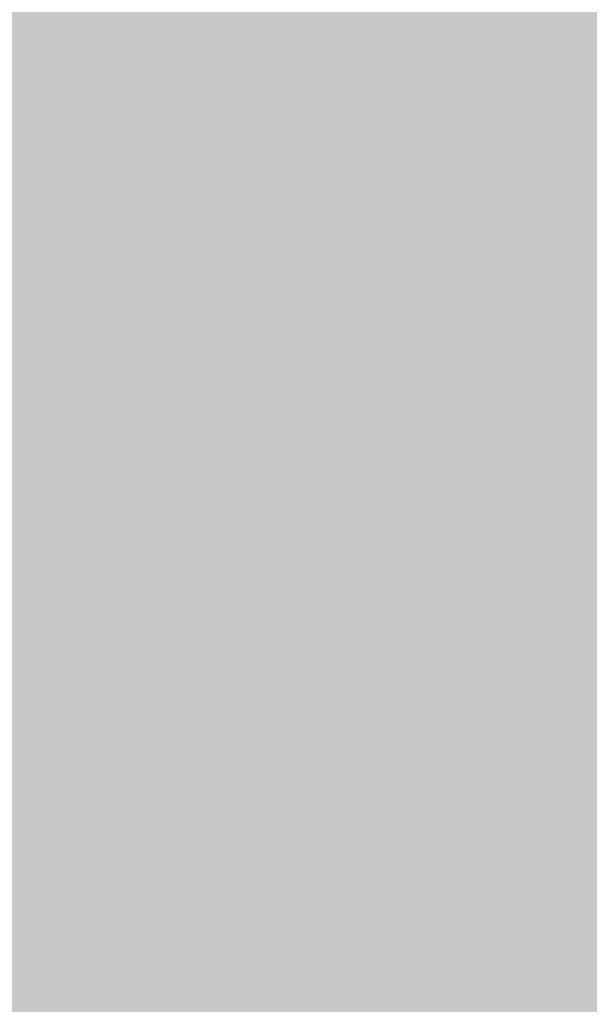
# Model space of a CAD drawing. Units: millimetres. Extents: x -22994 to 29398, y -19990 to 20176.
# Tile 82 of 135: x 226.355 to 227.437, y 85.199 to 87.071. Entities that reach past the tile are written whole.
import ezdxf
from ezdxf import colors
from ezdxf.entities.mleader import LeaderData, LeaderLine
from ezdxf.math import Vec2, Vec3

# ---------------------------------------------------------------- set-up
doc = ezdxf.new("R2010")
doc.units = ezdxf.units.MM
doc.header["$MEASUREMENT"] = 0
doc.layers.add('M-ANNO-TEXT', color=7, linetype='Continuous', lineweight=25)
doc.layers.add('M-DIMS', color=2, linetype='Continuous', lineweight=18)
doc.styles.get("Standard").update_dxf_attribs({"font": 'arial.ttf'})
doc.dimstyles.get("Standard").update_dxf_attribs({"dimtxt": 0.18, "dimasz": 10000, "dimexe": 0.18, "dimexo": 0.0625, "dimgap": 0.09, "dimtad": 0, "dimtih": 1, "dimtoh": 1, "dimdec": 0, "dimzin": 0, "dimdsep": 46, "dimtxsty": 'Standard', "dimcen": 0.09, "dimadec": 0, "dimazin": 0, "dimtfac": 1, "dimtdec": 0, "dimtofl": 0, "dimtmove": 0, "dimatfit": 3, "dimfxl": 1, "dimtolj": 1, "dimtzin": 0, "dimlwd": 30, "dimarcsym": 0})

# ---------------------------------------------------------------- blocks, each defined once
blk = doc.blocks.new('*D2')
at = {"layer": 'Defpoints', "color": 0, "transparency": 16777216}
for p in [(6.6773, 10.2713), (290.852, 10.2713), (290.852, -5.0787)]:
    blk.add_point(p, dxfattribs=at)
at = {"layer": 'M-DIMS', "color": 0, "lineweight": -2, "transparency": 16777216}
for p, q in [((6.6773, 10.2088), (6.6773, -5.2587)), ((290.852, 10.2088), (290.852, -5.2587))]:
    blk.add_line(p, q, dxfattribs=at)
at = {"layer": 'M-DIMS', "color": 0, "lineweight": 30, "transparency": 16777216}
for p, q in [((-9993.3227, -5.0787), (-19993.3227, -5.0787)), ((10290.852, -5.0787), (20290.852, -5.0787))]:
    blk.add_line(p, q, dxfattribs=at)
at = {"layer": 'M-DIMS', "color": 0, "transparency": 16777216}
for points in [[(-9993.3227, 1661.5879), (-9993.3227, -1671.7454), (6.6773, -5.0787)], [(10290.852, 1661.5879), (10290.852, -1671.7454), (290.852, -5.0787)]]:
    blk.add_solid(points, dxfattribs=at)
at = {"layer": 'M-DIMS', "color": 0, "transparency": 16777216, "insert": (148.7647, -5.0787), "char_height": 0.18, "attachment_point": 5}
blk.add_mtext('\\A1;284.2', dxfattribs=at)
blk = doc.blocks.new('*D3')
at = {"layer": 'Defpoints', "color": 0, "transparency": 16777216}
for p in [(110.2647, 204.1654), (110.2647, 176.3662), (95.8327, 127.967)]:
    blk.add_point(p, dxfattribs=at)
at = {"layer": 'M-DIMS', "color": 0, "lineweight": -2, "transparency": 16777216}
for p, q in [((95.8327, 128.0295), (95.8327, 204.3454)), ((110.2647, 176.4287), (110.2647, 204.3454))]:
    blk.add_line(p, q, dxfattribs=at)
at = {"layer": 'M-DIMS', "color": 0, "lineweight": 30, "transparency": 16777216}
for p, q in [((-9904.1673, 204.1654), (-19904.1673, 204.1654)), ((10110.2647, 204.1654), (20110.2647, 204.1654))]:
    blk.add_line(p, q, dxfattribs=at)
at = {"layer": 'M-DIMS', "color": 0, "transparency": 16777216}
for points in [[(-9904.1673, 1870.8321), (-9904.1673, -1462.5013), (95.8327, 204.1654)], [(10110.2647, 1870.8321), (10110.2647, -1462.5013), (110.2647, 204.1654)]]:
    blk.add_solid(points, dxfattribs=at)
at = {"layer": 'M-DIMS', "color": 0, "transparency": 16777216, "insert": (103.0487, 204.1654), "char_height": 0.18, "attachment_point": 5}
blk.add_mtext('\\A1;14.432', dxfattribs=at)
blk = doc.blocks.new('*D4')
at = {"layer": 'Defpoints', "color": 0, "transparency": 16777216}
for p in [(116.2647, 204.1654), (110.2647, 176.3662), (116.2647, 176.3662)]:
    blk.add_point(p, dxfattribs=at)
at = {"layer": 'M-DIMS', "color": 0, "lineweight": -2, "transparency": 16777216}
for p, q in [((110.2647, 176.4287), (110.2647, 204.3454)), ((116.2647, 176.4287), (116.2647, 204.3454))]:
    blk.add_line(p, q, dxfattribs=at)
at = {"layer": 'M-DIMS', "color": 0, "lineweight": 30, "transparency": 16777216}
for p, q in [((-9889.7353, 204.1654), (-19889.7353, 204.1654)), ((10116.2647, 204.1654), (20116.2647, 204.1654))]:
    blk.add_line(p, q, dxfattribs=at)
at = {"layer": 'M-DIMS', "color": 0, "transparency": 16777216}
for points in [[(-9889.7353, 1870.8321), (-9889.7353, -1462.5013), (110.2647, 204.1654)], [(10116.2647, 1870.8321), (10116.2647, -1462.5013), (116.2647, 204.1654)]]:
    blk.add_solid(points, dxfattribs=at)
at = {"layer": 'M-DIMS', "color": 0, "transparency": 16777216, "insert": (113.2647, 204.1654), "char_height": 0.18, "attachment_point": 5}
blk.add_mtext('\\A1;6', dxfattribs=at)
blk = doc.blocks.new('*D5')
at = {"layer": 'Defpoints', "color": 0, "transparency": 16777216}
for p in [(181.2647, 204.1654), (116.2647, 176.3662), (181.2647, 176.3662)]:
    blk.add_point(p, dxfattribs=at)
at = {"layer": 'M-DIMS', "color": 0, "lineweight": -2, "transparency": 16777216}
for p, q in [((116.2647, 176.4287), (116.2647, 204.3454)), ((181.2647, 176.4287), (181.2647, 204.3454))]:
    blk.add_line(p, q, dxfattribs=at)
at = {"layer": 'M-DIMS', "color": 0, "lineweight": 30, "transparency": 16777216}
for p, q in [((-9883.7353, 204.1654), (-19883.7353, 204.1654)), ((10181.2647, 204.1654), (20181.2647, 204.1654))]:
    blk.add_line(p, q, dxfattribs=at)
at = {"layer": 'M-DIMS', "color": 0, "transparency": 16777216}
for points in [[(-9883.7353, 1870.8321), (-9883.7353, -1462.5013), (116.2647, 204.1654)], [(10181.2647, 1870.8321), (10181.2647, -1462.5013), (181.2647, 204.1654)]]:
    blk.add_solid(points, dxfattribs=at)
at = {"layer": 'M-DIMS', "color": 0, "transparency": 16777216, "insert": (148.7647, 204.1654), "char_height": 0.18, "attachment_point": 5}
blk.add_mtext('\\A1;65', dxfattribs=at)
blk = doc.blocks.new('*D6')
at = {"layer": 'Defpoints', "color": 0, "transparency": 16777216}
for p in [(187.2647, 204.1654), (181.2647, 176.3662), (187.2647, 176.3662)]:
    blk.add_point(p, dxfattribs=at)
at = {"layer": 'M-DIMS', "color": 0, "lineweight": -2, "transparency": 16777216}
for p, q in [((181.2647, 176.4287), (181.2647, 204.3454)), ((187.2647, 176.4287), (187.2647, 204.3454))]:
    blk.add_line(p, q, dxfattribs=at)
at = {"layer": 'M-DIMS', "color": 0, "lineweight": 30, "transparency": 16777216}
for p, q in [((-9818.7353, 204.1654), (-19818.7353, 204.1654)), ((10187.2647, 204.1654), (20187.2647, 204.1654))]:
    blk.add_line(p, q, dxfattribs=at)
at = {"layer": 'M-DIMS', "color": 0, "transparency": 16777216}
for points in [[(-9818.7353, 1870.8321), (-9818.7353, -1462.5013), (181.2647, 204.1654)], [(10187.2647, 1870.8321), (10187.2647, -1462.5013), (187.2647, 204.1654)]]:
    blk.add_solid(points, dxfattribs=at)
at = {"layer": 'M-DIMS', "color": 0, "transparency": 16777216, "insert": (184.2647, 204.1654), "char_height": 0.18, "attachment_point": 5}
blk.add_mtext('\\A1;6', dxfattribs=at)
blk = doc.blocks.new('*D7')
at = {"layer": 'Defpoints', "color": 0, "transparency": 16777216}
for p in [(201.6967, 204.1654), (187.2647, 176.3662), (201.6967, 127.967)]:
    blk.add_point(p, dxfattribs=at)
at = {"layer": 'M-DIMS', "color": 0, "lineweight": -2, "transparency": 16777216}
for p, q in [((187.2647, 176.4287), (187.2647, 204.3454)), ((201.6967, 128.0295), (201.6967, 204.3454))]:
    blk.add_line(p, q, dxfattribs=at)
at = {"layer": 'M-DIMS', "color": 0, "lineweight": 30, "transparency": 16777216}
for p, q in [((-9812.7353, 204.1654), (-19812.7353, 204.1654)), ((10201.6967, 204.1654), (20201.6967, 204.1654))]:
    blk.add_line(p, q, dxfattribs=at)
at = {"layer": 'M-DIMS', "color": 0, "transparency": 16777216}
for points in [[(-9812.7353, 1870.8321), (-9812.7353, -1462.5013), (187.2647, 204.1654)], [(10201.6967, 1870.8321), (10201.6967, -1462.5013), (201.6967, 204.1654)]]:
    blk.add_solid(points, dxfattribs=at)
at = {"layer": 'M-DIMS', "color": 0, "transparency": 16777216, "insert": (194.4807, 204.1654), "char_height": 0.18, "attachment_point": 5}
blk.add_mtext('\\A1;14.432', dxfattribs=at)
blk = doc.blocks.new('*D8')
at = {"layer": 'Defpoints', "color": 0, "transparency": 16777216}
for p in [(227.6485, 204.1654), (227.6485, 146.7296), (201.6967, 127.967)]:
    blk.add_point(p, dxfattribs=at)
at = {"layer": 'M-DIMS', "color": 0, "lineweight": -2, "transparency": 16777216}
for p, q in [((201.6967, 128.0295), (201.6967, 204.3454)), ((227.6485, 146.7921), (227.6485, 204.3454))]:
    blk.add_line(p, q, dxfattribs=at)
at = {"layer": 'M-DIMS', "color": 0, "lineweight": 30, "transparency": 16777216}
for p, q in [((-9798.3033, 204.1654), (-19798.3033, 204.1654)), ((10227.6485, 204.1654), (20227.6485, 204.1654))]:
    blk.add_line(p, q, dxfattribs=at)
at = {"layer": 'M-DIMS', "color": 0, "transparency": 16777216}
for points in [[(-9798.3033, 1870.8321), (-9798.3033, -1462.5013), (201.6967, 204.1654)], [(10227.6485, 1870.8321), (10227.6485, -1462.5013), (227.6485, 204.1654)]]:
    blk.add_solid(points, dxfattribs=at)
at = {"layer": 'M-DIMS', "color": 0, "transparency": 16777216, "insert": (214.6726, 204.1654), "char_height": 0.18, "attachment_point": 5}
blk.add_mtext('\\A1;25.95', dxfattribs=at)
blk = doc.blocks.new('*D9')
at = {"layer": 'Defpoints', "color": 0, "transparency": 16777216}
for p in [(187.2647, 176.3662), (306.202, 176.3662), (290.852, 10.2713)]:
    blk.add_point(p, dxfattribs=at)
at = {"layer": 'M-DIMS', "color": 0, "lineweight": 30, "transparency": 16777216}
for p, q in [((306.202, 10176.3662), (306.202, 20176.3662)), ((306.202, -9989.7287), (306.202, -19989.7287))]:
    blk.add_line(p, q, dxfattribs=at)
at = {"layer": 'M-DIMS', "color": 0, "lineweight": -2, "transparency": 16777216}
for p, q in [((187.3272, 176.3662), (306.382, 176.3662)), ((290.9145, 10.2713), (306.382, 10.2713))]:
    blk.add_line(p, q, dxfattribs=at)
at = {"layer": 'M-DIMS', "color": 0, "transparency": 16777216}
for points in [[(-1360.4646, 10176.3662), (1972.8687, 10176.3662), (306.202, 176.3662)], [(-1360.4646, -9989.7287), (1972.8687, -9989.7287), (306.202, 10.2713)]]:
    blk.add_solid(points, dxfattribs=at)
at = {"layer": 'M-DIMS', "color": 0, "transparency": 16777216, "insert": (306.202, 93.3187), "char_height": 0.18, "attachment_point": 5}
blk.add_mtext('\\A1;166.1', dxfattribs=at)
blk = doc.blocks.new('*D10')
at = {"layer": 'Defpoints', "color": 0, "transparency": 16777216}
for p in [(125.6498, 136.0713), (133.3459, 136.0713), (133.3459, -5.0787)]:
    blk.add_point(p, dxfattribs=at)
at = {"layer": 'M-DIMS', "color": 0, "lineweight": -2, "transparency": 16777216}
for p, q in [((125.6498, 136.0088), (125.6498, -5.2587)), ((133.3459, 136.0088), (133.3459, -5.2587))]:
    blk.add_line(p, q, dxfattribs=at)
at = {"layer": 'M-DIMS', "color": 0, "lineweight": 30, "transparency": 16777216}
for p, q in [((-9874.3502, -5.0787), (-19874.3502, -5.0787)), ((10133.3459, -5.0787), (20133.3459, -5.0787))]:
    blk.add_line(p, q, dxfattribs=at)
at = {"layer": 'M-DIMS', "color": 0, "transparency": 16777216}
for points in [[(-9874.3502, 1661.5879), (-9874.3502, -1671.7454), (125.6498, -5.0787)], [(10133.3459, 1661.5879), (10133.3459, -1671.7454), (133.3459, -5.0787)]]:
    blk.add_solid(points, dxfattribs=at)
at = {"layer": 'M-DIMS', "color": 0, "transparency": 16777216, "insert": (129.4978, -5.0787), "char_height": 0.18, "attachment_point": 5}
blk.add_mtext('\\A1;7.696', dxfattribs=at)
blk = doc.blocks.new('*D11')
at = {"layer": 'Defpoints', "color": 0, "transparency": 16777216}
for p in [(133.3459, 136.0713), (135.6498, 136.0713), (135.6498, -5.0787)]:
    blk.add_point(p, dxfattribs=at)
at = {"layer": 'M-DIMS', "color": 0, "lineweight": -2, "transparency": 16777216}
for p, q in [((133.3459, 136.0088), (133.3459, -5.2587)), ((135.6498, 136.0088), (135.6498, -5.2587))]:
    blk.add_line(p, q, dxfattribs=at)
at = {"layer": 'M-DIMS', "color": 0, "lineweight": 30, "transparency": 16777216}
for p, q in [((-9866.6541, -5.0787), (-19866.6541, -5.0787)), ((10135.6498, -5.0787), (20135.6498, -5.0787))]:
    blk.add_line(p, q, dxfattribs=at)
at = {"layer": 'M-DIMS', "color": 0, "transparency": 16777216}
for points in [[(-9866.6541, 1661.5879), (-9866.6541, -1671.7454), (133.3459, -5.0787)], [(10135.6498, 1661.5879), (10135.6498, -1671.7454), (135.6498, -5.0787)]]:
    blk.add_solid(points, dxfattribs=at)
at = {"layer": 'M-DIMS', "color": 0, "transparency": 16777216, "insert": (134.4978, -5.0787), "char_height": 0.18, "attachment_point": 5}
blk.add_mtext('\\A1;2.304', dxfattribs=at)
blk = doc.blocks.new('*D12')
at = {"layer": 'Defpoints', "color": 0, "transparency": 16777216}
for p in [(135.6498, 136.0713), (145.6498, 136.0713), (145.6498, -5.0787)]:
    blk.add_point(p, dxfattribs=at)
at = {"layer": 'M-DIMS', "color": 0, "lineweight": -2, "transparency": 16777216}
for p, q in [((135.6498, 136.0088), (135.6498, -5.2587)), ((145.6498, 136.0088), (145.6498, -5.2587))]:
    blk.add_line(p, q, dxfattribs=at)
at = {"layer": 'M-DIMS', "color": 0, "lineweight": 30, "transparency": 16777216}
for p, q in [((-9864.3502, -5.0787), (-19864.3502, -5.0787)), ((10145.6498, -5.0787), (20145.6498, -5.0787))]:
    blk.add_line(p, q, dxfattribs=at)
at = {"layer": 'M-DIMS', "color": 0, "transparency": 16777216}
for points in [[(-9864.3502, 1661.5879), (-9864.3502, -1671.7454), (135.6498, -5.0787)], [(10145.6498, 1661.5879), (10145.6498, -1671.7454), (145.6498, -5.0787)]]:
    blk.add_solid(points, dxfattribs=at)
at = {"layer": 'M-DIMS', "color": 0, "transparency": 16777216, "insert": (140.6498, -5.0787), "char_height": 0.18, "attachment_point": 5}
blk.add_mtext('\\A1;10', dxfattribs=at)
blk = doc.blocks.new('*D13')
at = {"layer": 'Defpoints', "color": 0, "transparency": 16777216}
for p in [(145.6498, 136.0713), (155.6498, 136.0713), (155.6498, -5.0787)]:
    blk.add_point(p, dxfattribs=at)
at = {"layer": 'M-DIMS', "color": 0, "lineweight": -2, "transparency": 16777216}
for p, q in [((145.6498, 136.0088), (145.6498, -5.2587)), ((155.6498, 136.0088), (155.6498, -5.2587))]:
    blk.add_line(p, q, dxfattribs=at)
at = {"layer": 'M-DIMS', "color": 0, "lineweight": 30, "transparency": 16777216}
for p, q in [((-9854.3502, -5.0787), (-19854.3502, -5.0787)), ((10155.6498, -5.0787), (20155.6498, -5.0787))]:
    blk.add_line(p, q, dxfattribs=at)
at = {"layer": 'M-DIMS', "color": 0, "transparency": 16777216}
for points in [[(-9854.3502, 1661.5879), (-9854.3502, -1671.7454), (145.6498, -5.0787)], [(10155.6498, 1661.5879), (10155.6498, -1671.7454), (155.6498, -5.0787)]]:
    blk.add_solid(points, dxfattribs=at)
at = {"layer": 'M-DIMS', "color": 0, "transparency": 16777216, "insert": (150.6498, -5.0787), "char_height": 0.18, "attachment_point": 5}
blk.add_mtext('\\A1;10', dxfattribs=at)
blk = doc.blocks.new('*D14')
at = {"layer": 'Defpoints', "color": 0, "transparency": 16777216}
for p in [(155.6498, 136.0713), (165.6498, 136.0713), (165.6498, -5.0787)]:
    blk.add_point(p, dxfattribs=at)
at = {"layer": 'M-DIMS', "color": 0, "lineweight": -2, "transparency": 16777216}
for p, q in [((155.6498, 136.0088), (155.6498, -5.2587)), ((165.6498, 136.0088), (165.6498, -5.2587))]:
    blk.add_line(p, q, dxfattribs=at)
at = {"layer": 'M-DIMS', "color": 0, "lineweight": 30, "transparency": 16777216}
for p, q in [((-9844.3502, -5.0787), (-19844.3502, -5.0787)), ((10165.6498, -5.0787), (20165.6498, -5.0787))]:
    blk.add_line(p, q, dxfattribs=at)
at = {"layer": 'M-DIMS', "color": 0, "transparency": 16777216}
for points in [[(-9844.3502, 1661.5879), (-9844.3502, -1671.7454), (155.6498, -5.0787)], [(10165.6498, 1661.5879), (10165.6498, -1671.7454), (165.6498, -5.0787)]]:
    blk.add_solid(points, dxfattribs=at)
at = {"layer": 'M-DIMS', "color": 0, "transparency": 16777216, "insert": (160.6498, -5.0787), "char_height": 0.18, "attachment_point": 5}
blk.add_mtext('\\A1;10', dxfattribs=at)
blk = doc.blocks.new('*D15')
at = {"layer": 'Defpoints', "color": 0, "transparency": 16777216}
for p in [(173.3459, 154.788), (173.3459, 136.0713), (306.202, 136.0713)]:
    blk.add_point(p, dxfattribs=at)
at = {"layer": 'M-DIMS', "color": 0, "lineweight": 30, "transparency": 16777216}
for p, q in [((306.202, 10154.788), (306.202, 20154.788)), ((306.202, -9863.9287), (306.202, -19863.9287))]:
    blk.add_line(p, q, dxfattribs=at)
at = {"layer": 'M-DIMS', "color": 0, "lineweight": -2, "transparency": 16777216}
for p, q in [((173.4084, 154.788), (306.382, 154.788)), ((173.4084, 136.0713), (306.382, 136.0713))]:
    blk.add_line(p, q, dxfattribs=at)
at = {"layer": 'M-DIMS', "color": 0, "transparency": 16777216}
for points in [[(-1360.4646, 10154.788), (1972.8687, 10154.788), (306.202, 154.788)], [(-1360.4646, -9863.9287), (1972.8687, -9863.9287), (306.202, 136.0713)]]:
    blk.add_solid(points, dxfattribs=at)
at = {"layer": 'M-DIMS', "color": 0, "transparency": 16777216, "insert": (306.202, 145.4297), "char_height": 0.18, "attachment_point": 5}
blk.add_mtext('\\A1;18.717', dxfattribs=at)
blk = doc.blocks.new('*D16')
at = {"layer": 'Defpoints', "color": 0, "transparency": 16777216}
for p in [(120.1702, 204.1654), (110.4658, 48.0349), (120.1702, 48.0349)]:
    blk.add_point(p, dxfattribs=at)
at = {"layer": 'M-DIMS', "color": 0, "lineweight": -2, "transparency": 16777216}
for p, q in [((110.4658, 48.0974), (110.4658, 204.3454)), ((120.1702, 48.0974), (120.1702, 204.3454))]:
    blk.add_line(p, q, dxfattribs=at)
at = {"layer": 'M-DIMS', "color": 0, "lineweight": 30, "transparency": 16777216}
for p, q in [((-9889.5342, 204.1654), (-19889.5342, 204.1654)), ((10120.1702, 204.1654), (20120.1702, 204.1654))]:
    blk.add_line(p, q, dxfattribs=at)
at = {"layer": 'M-DIMS', "color": 0, "transparency": 16777216}
for points in [[(-9889.5342, 1870.8321), (-9889.5342, -1462.5013), (110.4658, 204.1654)], [(10120.1702, 1870.8321), (10120.1702, -1462.5013), (120.1702, 204.1654)]]:
    blk.add_solid(points, dxfattribs=at)
at = {"layer": 'M-DIMS', "color": 0, "transparency": 16777216, "insert": (115.318, 204.1654), "char_height": 0.18, "attachment_point": 5}
blk.add_mtext('\\A1;9.704', dxfattribs=at)
blk = doc.blocks.new('*D17')
at = {"layer": 'Defpoints', "color": 0, "transparency": 16777216}
for p in [(126.1702, 204.1654), (120.1702, 48.0349), (126.1702, 48.0349)]:
    blk.add_point(p, dxfattribs=at)
at = {"layer": 'M-DIMS', "color": 0, "lineweight": -2, "transparency": 16777216}
for p, q in [((120.1702, 48.0974), (120.1702, 204.3454)), ((126.1702, 48.0974), (126.1702, 204.3454))]:
    blk.add_line(p, q, dxfattribs=at)
at = {"layer": 'M-DIMS', "color": 0, "lineweight": 30, "transparency": 16777216}
for p, q in [((-9879.8298, 204.1654), (-19879.8298, 204.1654)), ((10126.1702, 204.1654), (20126.1702, 204.1654))]:
    blk.add_line(p, q, dxfattribs=at)
at = {"layer": 'M-DIMS', "color": 0, "transparency": 16777216}
for points in [[(-9879.8298, 1870.8321), (-9879.8298, -1462.5013), (120.1702, 204.1654)], [(10126.1702, 1870.8321), (10126.1702, -1462.5013), (126.1702, 204.1654)]]:
    blk.add_solid(points, dxfattribs=at)
at = {"layer": 'M-DIMS', "color": 0, "transparency": 16777216, "insert": (123.1702, 204.1654), "char_height": 0.18, "attachment_point": 5}
blk.add_mtext('\\A1;6', dxfattribs=at)
blk = doc.blocks.new('*D18')
at = {"layer": 'Defpoints', "color": 0, "transparency": 16777216}
for p in [(132.1702, 204.1654), (126.1702, 48.0349), (132.1702, 48.0349)]:
    blk.add_point(p, dxfattribs=at)
at = {"layer": 'M-DIMS', "color": 0, "lineweight": -2, "transparency": 16777216}
for p, q in [((126.1702, 48.0974), (126.1702, 204.3454)), ((132.1702, 48.0974), (132.1702, 204.3454))]:
    blk.add_line(p, q, dxfattribs=at)
at = {"layer": 'M-DIMS', "color": 0, "lineweight": 30, "transparency": 16777216}
for p, q in [((-9873.8298, 204.1654), (-19873.8298, 204.1654)), ((10132.1702, 204.1654), (20132.1702, 204.1654))]:
    blk.add_line(p, q, dxfattribs=at)
at = {"layer": 'M-DIMS', "color": 0, "transparency": 16777216}
for points in [[(-9873.8298, 1870.8321), (-9873.8298, -1462.5013), (126.1702, 204.1654)], [(10132.1702, 1870.8321), (10132.1702, -1462.5013), (132.1702, 204.1654)]]:
    blk.add_solid(points, dxfattribs=at)
at = {"layer": 'M-DIMS', "color": 0, "transparency": 16777216, "insert": (129.1702, 204.1654), "char_height": 0.18, "attachment_point": 5}
blk.add_mtext('\\A1;6', dxfattribs=at)
blk = doc.blocks.new('*D19')
at = {"layer": 'Defpoints', "color": 0, "transparency": 16777216}
for p in [(138.1702, 204.1654), (132.1702, 48.0349), (138.1702, 48.0349)]:
    blk.add_point(p, dxfattribs=at)
at = {"layer": 'M-DIMS', "color": 0, "lineweight": -2, "transparency": 16777216}
for p, q in [((132.1702, 48.0974), (132.1702, 204.3454)), ((138.1702, 48.0974), (138.1702, 204.3454))]:
    blk.add_line(p, q, dxfattribs=at)
at = {"layer": 'M-DIMS', "color": 0, "lineweight": 30, "transparency": 16777216}
for p, q in [((-9867.8298, 204.1654), (-19867.8298, 204.1654)), ((10138.1702, 204.1654), (20138.1702, 204.1654))]:
    blk.add_line(p, q, dxfattribs=at)
at = {"layer": 'M-DIMS', "color": 0, "transparency": 16777216}
for points in [[(-9867.8298, 1870.8321), (-9867.8298, -1462.5013), (132.1702, 204.1654)], [(10138.1702, 1870.8321), (10138.1702, -1462.5013), (138.1702, 204.1654)]]:
    blk.add_solid(points, dxfattribs=at)
at = {"layer": 'M-DIMS', "color": 0, "transparency": 16777216, "insert": (135.1702, 204.1654), "char_height": 0.18, "attachment_point": 5}
blk.add_mtext('\\A1;6', dxfattribs=at)
blk = doc.blocks.new('*D20')
at = {"layer": 'Defpoints', "color": 0, "transparency": 16777216}
for p in [(144.1702, 204.1654), (138.1702, 48.0349), (144.1702, 48.0349)]:
    blk.add_point(p, dxfattribs=at)
at = {"layer": 'M-DIMS', "color": 0, "lineweight": -2, "transparency": 16777216}
for p, q in [((138.1702, 48.0974), (138.1702, 204.3454)), ((144.1702, 48.0974), (144.1702, 204.3454))]:
    blk.add_line(p, q, dxfattribs=at)
at = {"layer": 'M-DIMS', "color": 0, "lineweight": 30, "transparency": 16777216}
for p, q in [((-9861.8298, 204.1654), (-19861.8298, 204.1654)), ((10144.1702, 204.1654), (20144.1702, 204.1654))]:
    blk.add_line(p, q, dxfattribs=at)
at = {"layer": 'M-DIMS', "color": 0, "transparency": 16777216}
for points in [[(-9861.8298, 1870.8321), (-9861.8298, -1462.5013), (138.1702, 204.1654)], [(10144.1702, 1870.8321), (10144.1702, -1462.5013), (144.1702, 204.1654)]]:
    blk.add_solid(points, dxfattribs=at)
at = {"layer": 'M-DIMS', "color": 0, "transparency": 16777216, "insert": (141.1702, 204.1654), "char_height": 0.18, "attachment_point": 5}
blk.add_mtext('\\A1;6', dxfattribs=at)
blk = doc.blocks.new('*D21')
at = {"layer": 'Defpoints', "color": 0, "transparency": 16777216}
for p in [(149.1157, 204.1654), (144.1702, 48.0349), (149.1157, 48.0349)]:
    blk.add_point(p, dxfattribs=at)
at = {"layer": 'M-DIMS', "color": 0, "lineweight": -2, "transparency": 16777216}
for p, q in [((144.1702, 48.0974), (144.1702, 204.3454)), ((149.1157, 48.0974), (149.1157, 204.3454))]:
    blk.add_line(p, q, dxfattribs=at)
at = {"layer": 'M-DIMS', "color": 0, "lineweight": 30, "transparency": 16777216}
for p, q in [((-9855.8298, 204.1654), (-19855.8298, 204.1654)), ((10149.1157, 204.1654), (20149.1157, 204.1654))]:
    blk.add_line(p, q, dxfattribs=at)
at = {"layer": 'M-DIMS', "color": 0, "transparency": 16777216}
for points in [[(-9855.8298, 1870.8321), (-9855.8298, -1462.5013), (144.1702, 204.1654)], [(10149.1157, 1870.8321), (10149.1157, -1462.5013), (149.1157, 204.1654)]]:
    blk.add_solid(points, dxfattribs=at)
at = {"layer": 'M-DIMS', "color": 0, "transparency": 16777216, "insert": (146.6429, 204.1654), "char_height": 0.18, "attachment_point": 5}
blk.add_mtext('\\A1;4.945', dxfattribs=at)
blk = doc.blocks.new('*D22')
at = {"layer": 'Defpoints', "color": 0, "transparency": 16777216}
for p in [(149.1157, 30.9895), (155.1157, 30.9895), (155.1157, -5.0787)]:
    blk.add_point(p, dxfattribs=at)
at = {"layer": 'M-DIMS', "color": 0, "lineweight": -2, "transparency": 16777216}
for p, q in [((149.1157, 30.927), (149.1157, -5.2587)), ((155.1157, 30.927), (155.1157, -5.2587))]:
    blk.add_line(p, q, dxfattribs=at)
at = {"layer": 'M-DIMS', "color": 0, "lineweight": 30, "transparency": 16777216}
for p, q in [((-9850.8843, -5.0787), (-19850.8843, -5.0787)), ((10155.1157, -5.0787), (20155.1157, -5.0787))]:
    blk.add_line(p, q, dxfattribs=at)
at = {"layer": 'M-DIMS', "color": 0, "transparency": 16777216}
for points in [[(-9850.8843, 1661.5879), (-9850.8843, -1671.7454), (149.1157, -5.0787)], [(10155.1157, 1661.5879), (10155.1157, -1671.7454), (155.1157, -5.0787)]]:
    blk.add_solid(points, dxfattribs=at)
at = {"layer": 'M-DIMS', "color": 0, "transparency": 16777216, "insert": (152.1157, -5.0787), "char_height": 0.18, "attachment_point": 5}
blk.add_mtext('\\A1;6', dxfattribs=at)
blk = doc.blocks.new('*D23')
at = {"layer": 'Defpoints', "color": 0, "transparency": 16777216}
for p in [(155.1157, 30.9895), (161.1157, 30.9895), (161.1157, -5.0787)]:
    blk.add_point(p, dxfattribs=at)
at = {"layer": 'M-DIMS', "color": 0, "lineweight": -2, "transparency": 16777216}
for p, q in [((155.1157, 30.927), (155.1157, -5.2587)), ((161.1157, 30.927), (161.1157, -5.2587))]:
    blk.add_line(p, q, dxfattribs=at)
at = {"layer": 'M-DIMS', "color": 0, "lineweight": 30, "transparency": 16777216}
for p, q in [((-9844.8843, -5.0787), (-19844.8843, -5.0787)), ((10161.1157, -5.0787), (20161.1157, -5.0787))]:
    blk.add_line(p, q, dxfattribs=at)
at = {"layer": 'M-DIMS', "color": 0, "transparency": 16777216}
for points in [[(-9844.8843, 1661.5879), (-9844.8843, -1671.7454), (155.1157, -5.0787)], [(10161.1157, 1661.5879), (10161.1157, -1671.7454), (161.1157, -5.0787)]]:
    blk.add_solid(points, dxfattribs=at)
at = {"layer": 'M-DIMS', "color": 0, "transparency": 16777216, "insert": (158.1157, -5.0787), "char_height": 0.18, "attachment_point": 5}
blk.add_mtext('\\A1;6', dxfattribs=at)
blk = doc.blocks.new('*D24')
at = {"layer": 'Defpoints', "color": 0, "transparency": 16777216}
for p in [(161.1157, 30.9895), (166.4387, 30.9895), (166.4387, -5.0787)]:
    blk.add_point(p, dxfattribs=at)
at = {"layer": 'M-DIMS', "color": 0, "lineweight": -2, "transparency": 16777216}
for p, q in [((161.1157, 30.927), (161.1157, -5.2587)), ((166.4387, 30.927), (166.4387, -5.2587))]:
    blk.add_line(p, q, dxfattribs=at)
at = {"layer": 'M-DIMS', "color": 0, "lineweight": 30, "transparency": 16777216}
for p, q in [((-9838.8843, -5.0787), (-19838.8843, -5.0787)), ((10166.4387, -5.0787), (20166.4387, -5.0787))]:
    blk.add_line(p, q, dxfattribs=at)
at = {"layer": 'M-DIMS', "color": 0, "transparency": 16777216}
for points in [[(-9838.8843, 1661.5879), (-9838.8843, -1671.7454), (161.1157, -5.0787)], [(10166.4387, 1661.5879), (10166.4387, -1671.7454), (166.4387, -5.0787)]]:
    blk.add_solid(points, dxfattribs=at)
at = {"layer": 'M-DIMS', "color": 0, "transparency": 16777216, "insert": (163.7772, -5.0787), "char_height": 0.18, "attachment_point": 5}
blk.add_mtext('\\A1;5.323', dxfattribs=at)
blk = doc.blocks.new('*D25')
at = {"layer": 'Defpoints', "color": 0, "transparency": 16777216}
for p in [(166.4387, 30.9895), (172.4387, 30.9895), (172.4387, -5.0787)]:
    blk.add_point(p, dxfattribs=at)
at = {"layer": 'M-DIMS', "color": 0, "lineweight": -2, "transparency": 16777216}
for p, q in [((166.4387, 30.927), (166.4387, -5.2587)), ((172.4387, 30.927), (172.4387, -5.2587))]:
    blk.add_line(p, q, dxfattribs=at)
at = {"layer": 'M-DIMS', "color": 0, "lineweight": 30, "transparency": 16777216}
for p, q in [((-9833.5613, -5.0787), (-19833.5613, -5.0787)), ((10172.4387, -5.0787), (20172.4387, -5.0787))]:
    blk.add_line(p, q, dxfattribs=at)
at = {"layer": 'M-DIMS', "color": 0, "transparency": 16777216}
for points in [[(-9833.5613, 1661.5879), (-9833.5613, -1671.7454), (166.4387, -5.0787)], [(10172.4387, 1661.5879), (10172.4387, -1671.7454), (172.4387, -5.0787)]]:
    blk.add_solid(points, dxfattribs=at)
at = {"layer": 'M-DIMS', "color": 0, "transparency": 16777216, "insert": (169.4387, -5.0787), "char_height": 0.18, "attachment_point": 5}
blk.add_mtext('\\A1;6', dxfattribs=at)
blk = doc.blocks.new('*D26')
at = {"layer": 'Defpoints', "color": 0, "transparency": 16777216}
for p in [(172.4387, 30.9895), (178.4387, 30.9895), (178.4387, -5.0787)]:
    blk.add_point(p, dxfattribs=at)
at = {"layer": 'M-DIMS', "color": 0, "lineweight": -2, "transparency": 16777216}
for p, q in [((172.4387, 30.927), (172.4387, -5.2587)), ((178.4387, 30.927), (178.4387, -5.2587))]:
    blk.add_line(p, q, dxfattribs=at)
at = {"layer": 'M-DIMS', "color": 0, "lineweight": 30, "transparency": 16777216}
for p, q in [((-9827.5613, -5.0787), (-19827.5613, -5.0787)), ((10178.4387, -5.0787), (20178.4387, -5.0787))]:
    blk.add_line(p, q, dxfattribs=at)
at = {"layer": 'M-DIMS', "color": 0, "transparency": 16777216}
for points in [[(-9827.5613, 1661.5879), (-9827.5613, -1671.7454), (172.4387, -5.0787)], [(10178.4387, 1661.5879), (10178.4387, -1671.7454), (178.4387, -5.0787)]]:
    blk.add_solid(points, dxfattribs=at)
at = {"layer": 'M-DIMS', "color": 0, "transparency": 16777216, "insert": (175.4387, -5.0787), "char_height": 0.18, "attachment_point": 5}
blk.add_mtext('\\A1;6', dxfattribs=at)
blk = doc.blocks.new('*D27')
at = {"layer": 'Defpoints', "color": 0, "transparency": 16777216}
for p in [(178.4387, 30.9895), (188.1175, 30.9895), (188.1175, -5.0787)]:
    blk.add_point(p, dxfattribs=at)
at = {"layer": 'M-DIMS', "color": 0, "lineweight": -2, "transparency": 16777216}
for p, q in [((178.4387, 30.927), (178.4387, -5.2587)), ((188.1175, 30.927), (188.1175, -5.2587))]:
    blk.add_line(p, q, dxfattribs=at)
at = {"layer": 'M-DIMS', "color": 0, "lineweight": 30, "transparency": 16777216}
for p, q in [((-9821.5613, -5.0787), (-19821.5613, -5.0787)), ((10188.1175, -5.0787), (20188.1175, -5.0787))]:
    blk.add_line(p, q, dxfattribs=at)
at = {"layer": 'M-DIMS', "color": 0, "transparency": 16777216}
for points in [[(-9821.5613, 1661.5879), (-9821.5613, -1671.7454), (178.4387, -5.0787)], [(10188.1175, 1661.5879), (10188.1175, -1671.7454), (188.1175, -5.0787)]]:
    blk.add_solid(points, dxfattribs=at)
at = {"layer": 'M-DIMS', "color": 0, "transparency": 16777216, "insert": (183.2781, -5.0787), "char_height": 0.18, "attachment_point": 5}
blk.add_mtext('\\A1;9.679', dxfattribs=at)
blk = doc.blocks.new('*D28')
at = {"layer": 'Defpoints', "color": 0, "transparency": 16777216}
for p in [(188.1175, 48.0349), (306.202, 48.0349), (188.1175, 30.9895)]:
    blk.add_point(p, dxfattribs=at)
at = {"layer": 'M-DIMS', "color": 0, "lineweight": 30, "transparency": 16777216}
for p, q in [((306.202, 10048.0349), (306.202, 20048.0349)), ((306.202, -9969.0105), (306.202, -19969.0105))]:
    blk.add_line(p, q, dxfattribs=at)
at = {"layer": 'M-DIMS', "color": 0, "lineweight": -2, "transparency": 16777216}
for p, q in [((188.18, 48.0349), (306.382, 48.0349)), ((188.18, 30.9895), (306.382, 30.9895))]:
    blk.add_line(p, q, dxfattribs=at)
at = {"layer": 'M-DIMS', "color": 0, "transparency": 16777216}
for points in [[(-1360.4646, 10048.0349), (1972.8687, 10048.0349), (306.202, 48.0349)], [(-1360.4646, -9969.0105), (1972.8687, -9969.0105), (306.202, 30.9895)]]:
    blk.add_solid(points, dxfattribs=at)
at = {"layer": 'M-DIMS', "color": 0, "transparency": 16777216, "insert": (306.202, 39.5122), "char_height": 0.18, "attachment_point": 5}
blk.add_mtext('\\A1;17.045', dxfattribs=at)
blk = doc.blocks.new('*D29')
at = {"layer": 'Defpoints', "color": 0, "transparency": 16777216}
for p in [(36.8006, 80.045), (64.0296, 80.045)]:
    blk.add_point(p, dxfattribs=at)
at = {"layer": 'M-DIMS', "color": 0, "lineweight": -2, "transparency": 16777216}
for p, q in [((50.4151, 79.955), (50.4151, 80.135)), ((50.3251, 80.045), (50.5051, 80.045))]:
    blk.add_line(p, q, dxfattribs=at)
at = {"layer": 'M-DIMS', "color": 0, "lineweight": 30, "transparency": 16777216}
blk.add_line((20064.0296, 80.0303), (10064.0296, 80.0377), dxfattribs=at)
at = {"layer": 'M-DIMS', "color": 0, "transparency": 16777216}
blk.add_solid([(10064.0309, 1746.7043), (10064.0284, -1586.629), (64.0296, 80.045)], dxfattribs=at)
at = {"layer": 'M-DIMS', "color": 0, "transparency": 16777216, "insert": (20064.5213, 80.0303), "char_height": 0.18, "attachment_point": 5}
blk.add_mtext('\\A1;∅27.23', dxfattribs=at)
blk = doc.blocks.new('*D30')
at = {"layer": 'Defpoints', "color": 0, "transparency": 16777216}
for p in [(216.3148, 146.7291), (238.9821, 146.73)]:
    blk.add_point(p, dxfattribs=at)
at = {"layer": 'M-DIMS', "color": 0, "lineweight": 30, "transparency": 16777216}
blk.add_line((20238.9821, 147.4959), (10238.9821, 147.1129), dxfattribs=at)
at = {"layer": 'M-DIMS', "color": 0, "lineweight": -2, "transparency": 16777216}
for p, q in [((227.6485, 146.6396), (227.6485, 146.8196)), ((227.5585, 146.7296), (227.7385, 146.7296))]:
    blk.add_line(p, q, dxfattribs=at)
at = {"layer": 'M-DIMS', "color": 0, "transparency": 16777216}
blk.add_solid([(10238.9183, 1813.7796), (10239.0459, -1519.5537), (238.9821, 146.73)], dxfattribs=at)
at = {"layer": 'M-DIMS', "color": 0, "transparency": 16777216, "insert": (20239.5436, 147.4959), "char_height": 0.18, "attachment_point": 5}
blk.add_mtext('\\A1;∅22.667', dxfattribs=at)
blk = doc.blocks.new('*D31')
at = {"layer": 'Defpoints', "color": 0, "transparency": 16777216}
for p in [(223.1641, 146.7291), (232.1328, 146.73)]:
    blk.add_point(p, dxfattribs=at)
at = {"layer": 'M-DIMS', "color": 0, "lineweight": 30, "transparency": 16777216}
blk.add_line((20232.1327, 148.6656), (10232.1328, 147.6978), dxfattribs=at)
at = {"layer": 'M-DIMS', "color": 0, "lineweight": -2, "transparency": 16777216}
for p, q in [((227.6485, 146.6396), (227.6485, 146.8196)), ((227.5585, 146.7296), (227.7385, 146.7296))]:
    blk.add_line(p, q, dxfattribs=at)
at = {"layer": 'M-DIMS', "color": 0, "transparency": 16777216}
blk.add_solid([(10231.9715, 1814.3645), (10232.2941, -1518.9688), (232.1328, 146.73)], dxfattribs=at)
at = {"layer": 'M-DIMS', "color": 0, "transparency": 16777216, "insert": (20232.6245, 148.6656), "char_height": 0.18, "attachment_point": 5}
blk.add_mtext('\\A1;∅8.969', dxfattribs=at)
blk = doc.blocks.new('*D36')
at = {"layer": 'Defpoints', "color": 0, "transparency": 16777216}
for p in [(46.39, 31.3035), (46.3875, 26.5934)]:
    blk.add_point(p, dxfattribs=at)
at = {"layer": 'M-DIMS', "color": 0, "lineweight": 30, "transparency": 16777216}
for p, q in [((57.1499, 20031.3006), (51.77, 10031.302)), ((10057.1499, 20031.3006), (57.1499, 20031.3006))]:
    blk.add_line(p, q, dxfattribs=at)
at = {"layer": 'M-DIMS', "color": 0, "lineweight": -2, "transparency": 16777216}
for p, q in [((46.3887, 28.8585), (46.3887, 29.0385)), ((46.2987, 28.9485), (46.4787, 28.9485))]:
    blk.add_line(p, q, dxfattribs=at)
at = {"layer": 'M-DIMS', "color": 0, "transparency": 16777216}
blk.add_solid([(-1614.8965, 10032.1987), (1718.4364, 10030.4054), (46.39, 31.3035)], dxfattribs=at)
at = {"layer": 'M-DIMS', "color": 0, "transparency": 16777216, "insert": (10057.5542, 20031.3006), "char_height": 0.18, "attachment_point": 5}
blk.add_mtext('\\A1;∅4.71', dxfattribs=at)
blk = doc.blocks.new('*D37')
at = {"layer": 'Defpoints', "color": 0, "transparency": 16777216}
for p in [(54.8343, 118.6145), (59.4936, 118.614)]:
    blk.add_point(p, dxfattribs=at)
at = {"layer": 'M-DIMS', "color": 0, "lineweight": -2, "transparency": 16777216}
for p, q in [((57.1639, 118.5243), (57.1639, 118.7043)), ((57.0739, 118.6143), (57.2539, 118.6143))]:
    blk.add_line(p, q, dxfattribs=at)
at = {"layer": 'M-DIMS', "color": 0, "lineweight": 30, "transparency": 16777216}
blk.add_line((20059.4934, 116.2531), (10059.4935, 117.4336), dxfattribs=at)
at = {"layer": 'M-DIMS', "color": 0, "transparency": 16777216}
blk.add_solid([(10059.6902, 1784.1002), (10059.2968, -1549.2331), (59.4936, 118.614)], dxfattribs=at)
at = {"layer": 'M-DIMS', "color": 0, "transparency": 16777216, "insert": (20059.9852, 116.2531), "char_height": 0.18, "attachment_point": 5}
blk.add_mtext('\\A1;∅4.659', dxfattribs=at)

msp = doc.modelspace()

# ---------------------------------------------------------------- dimensions: what is measured, and where the dimension line sits
at = {"layer": 'M-DIMS'}
for base, p1, p2, override, picture, middle in [((306.202, 176.3662), (290.852, 10.2713), (187.2647, 176.3662), {"dimdec": 1, "dimlfac": 1, "dimrnd": 0, "dimzin": 0, "dimdsep": 46, "dimlunit": 2}, '*D9', (306.202, 93.3187)), ((306.202, 136.0713), (173.3459, 154.788), (173.3459, 136.0713), {"dimdec": 3, "dimlfac": 1, "dimrnd": 0, "dimzin": 0, "dimdsep": 46, "dimlunit": 2}, '*D15', (306.202, 145.4297)), ((306.202, 48.0349), (188.1175, 30.9895), (188.1175, 48.0349), {"dimdec": 3, "dimlfac": 1, "dimrnd": 0, "dimzin": 0, "dimdsep": 46, "dimlunit": 2}, '*D28', (306.202, 39.5122))]:
    dim = msp.add_linear_dim(base=base, p1=p1, p2=p2, angle=90, dimstyle='Standard', override=override, dxfattribs=at)
    dim.commit()
    dim.dimension.update_dxf_attribs({"geometry": picture, "text_midpoint": middle})
for p1, p2, override, picture, middle in [((46.3875, 26.5934), (46.39, 31.3035), {"dimdec": 2, "dimlfac": 1, "dimrnd": 0, "dimzin": 0, "dimdsep": 46, "dimlunit": 2}, '*D36', (10057.5542, 20031.3006)), ((223.1641, 146.7291), (232.1328, 146.73), {"dimdec": 3, "dimlfac": 1, "dimrnd": 0, "dimzin": 0, "dimdsep": 46, "dimlunit": 2}, '*D31', (20232.1327, 148.6656)), ((216.3148, 146.7291), (238.9821, 146.73), {"dimdec": 3, "dimlfac": 1, "dimrnd": 0, "dimzin": 0, "dimdsep": 46, "dimlunit": 2}, '*D30', (20238.9821, 147.4959))]:
    dim = msp.add_diameter_dim_2p(p1=p1, p2=p2, dimstyle='Standard', override=override, dxfattribs=at)
    dim.commit()
    dim.dimension.update_dxf_attribs({"geometry": picture, "text_midpoint": middle, "dimtype": 163})
for base, p1, p2, override, picture, middle in [((110.2647, 204.1654), (95.8327, 127.967), (110.2647, 176.3662), {"dimdec": 3, "dimlfac": 1, "dimrnd": 0, "dimzin": 0, "dimdsep": 46, "dimlunit": 2}, '*D3', (103.0487, 204.1654)), ((116.2647, 204.1654), (110.2647, 176.3662), (116.2647, 176.3662), {"dimdec": 0, "dimlfac": 1, "dimrnd": 0, "dimzin": 0, "dimdsep": 46, "dimlunit": 2}, '*D4', (113.2647, 204.1654)), ((120.1702, 204.1654), (110.4658, 48.0349), (120.1702, 48.0349), {"dimdec": 3, "dimlfac": 1, "dimrnd": 0, "dimzin": 0, "dimdsep": 46, "dimlunit": 2}, '*D16', (115.318, 204.1654)), ((181.2647, 204.1654), (116.2647, 176.3662), (181.2647, 176.3662), {"dimdec": 0, "dimlfac": 1, "dimrnd": 0, "dimzin": 0, "dimdsep": 46, "dimlunit": 2}, '*D5', (148.7647, 204.1654)), ((126.1702, 204.1654), (120.1702, 48.0349), (126.1702, 48.0349), {"dimdec": 0, "dimlfac": 1, "dimrnd": 0, "dimzin": 0, "dimdsep": 46, "dimlunit": 2}, '*D17', (123.1702, 204.1654)), ((132.1702, 204.1654), (126.1702, 48.0349), (132.1702, 48.0349), {"dimdec": 0, "dimlfac": 1, "dimrnd": 0, "dimzin": 0, "dimdsep": 46, "dimlunit": 2}, '*D18', (129.1702, 204.1654)), ((138.1702, 204.1654), (132.1702, 48.0349), (138.1702, 48.0349), {"dimdec": 0, "dimlfac": 1, "dimrnd": 0, "dimzin": 0, "dimdsep": 46, "dimlunit": 2}, '*D19', (135.1702, 204.1654)), ((144.1702, 204.1654), (138.1702, 48.0349), (144.1702, 48.0349), {"dimdec": 0, "dimlfac": 1, "dimrnd": 0, "dimzin": 0, "dimdsep": 46, "dimlunit": 2}, '*D20', (141.1702, 204.1654)), ((149.11567, 204.16539), (144.17023, 48.03494), (149.11567, 48.03494), {"dimdec": 3, "dimlfac": 1, "dimrnd": 0, "dimzin": 0, "dimdsep": 46, "dimlunit": 2}, '*D21', (146.64295, 204.16539)), ((187.2647, 204.1654), (181.2647, 176.3662), (187.2647, 176.3662), {"dimdec": 0, "dimlfac": 1, "dimrnd": 0, "dimzin": 0, "dimdsep": 46, "dimlunit": 2}, '*D6', (184.2647, 204.1654)), ((201.6967, 204.1654), (187.2647, 176.3662), (201.6967, 127.967), {"dimdec": 3, "dimlfac": 1, "dimrnd": 0, "dimzin": 0, "dimdsep": 46, "dimlunit": 2}, '*D7', (194.4807, 204.1654)), ((227.6485, 204.1654), (201.6967, 127.967), (227.6485, 146.7296), {"dimdec": 2, "dimlfac": 1, "dimrnd": 0, "dimzin": 0, "dimdsep": 46, "dimlunit": 2}, '*D8', (214.6726, 204.1654)), ((290.852, -5.0787), (6.6773, 10.2713), (290.852, 10.2713), {"dimdec": 1, "dimlfac": 1, "dimrnd": 0, "dimzin": 0, "dimdsep": 46, "dimlunit": 2}, '*D2', (148.7647, -5.0787)), ((133.3459, -5.0787), (125.6498, 136.0713), (133.3459, 136.0713), {"dimdec": 3, "dimlfac": 1, "dimrnd": 0, "dimzin": 0, "dimdsep": 46, "dimlunit": 2}, '*D10', (129.4978, -5.0787)), ((135.6498, -5.0787), (133.3459, 136.0713), (135.6498, 136.0713), {"dimdec": 3, "dimlfac": 1, "dimrnd": 0, "dimzin": 0, "dimdsep": 46, "dimlunit": 2}, '*D11', (134.4978, -5.0787)), ((145.6498, -5.0787), (135.6498, 136.0713), (145.6498, 136.0713), {"dimdec": 0, "dimlfac": 1, "dimrnd": 0, "dimzin": 0, "dimdsep": 46, "dimlunit": 2}, '*D12', (140.6498, -5.0787)), ((155.6498, -5.0787), (145.6498, 136.0713), (155.6498, 136.0713), {"dimdec": 0, "dimlfac": 1, "dimrnd": 0, "dimzin": 0, "dimdsep": 46, "dimlunit": 2}, '*D13', (150.6498, -5.0787)), ((155.1157, -5.0787), (149.1157, 30.9895), (155.1157, 30.9895), {"dimdec": 0, "dimlfac": 1, "dimrnd": 0, "dimzin": 0, "dimdsep": 46, "dimlunit": 2}, '*D22', (152.1157, -5.0787)), ((161.1157, -5.0787), (155.1157, 30.9895), (161.1157, 30.9895), {"dimdec": 0, "dimlfac": 1, "dimrnd": 0, "dimzin": 0, "dimdsep": 46, "dimlunit": 2}, '*D23', (158.1157, -5.0787)), ((165.6498, -5.0787), (155.6498, 136.0713), (165.6498, 136.0713), {"dimdec": 0, "dimlfac": 1, "dimrnd": 0, "dimzin": 0, "dimdsep": 46, "dimlunit": 2}, '*D14', (160.6498, -5.0787)), ((166.4387, -5.0787), (161.1157, 30.9895), (166.4387, 30.9895), {"dimdec": 3, "dimlfac": 1, "dimrnd": 0, "dimzin": 0, "dimdsep": 46, "dimlunit": 2}, '*D24', (163.7772, -5.0787)), ((172.4387, -5.0787), (166.4387, 30.9895), (172.4387, 30.9895), {"dimdec": 0, "dimlfac": 1, "dimrnd": 0, "dimzin": 0, "dimdsep": 46, "dimlunit": 2}, '*D25', (169.4387, -5.0787)), ((178.4387, -5.0787), (172.4387, 30.9895), (178.4387, 30.9895), {"dimdec": 0, "dimlfac": 1, "dimrnd": 0, "dimzin": 0, "dimdsep": 46, "dimlunit": 2}, '*D26', (175.4387, -5.0787)), ((188.1175, -5.0787), (178.4387, 30.9895), (188.1175, 30.9895), {"dimdec": 3, "dimlfac": 1, "dimrnd": 0, "dimzin": 0, "dimdsep": 46, "dimlunit": 2}, '*D27', (183.2781, -5.0787))]:
    dim = msp.add_linear_dim(base=base, p1=p1, p2=p2, dimstyle='Standard', override=override, dxfattribs=at)
    dim.commit()
    dim.dimension.update_dxf_attribs({"geometry": picture, "text_midpoint": middle})
for p1, p2, override, picture, middle in [((54.8343, 118.6145), (59.4936, 118.614), {"dimdec": 3, "dimlfac": 1, "dimrnd": 0, "dimzin": 0, "dimdsep": 46, "dimlunit": 2}, '*D37', (20059.4934, 116.2531)), ((36.8006, 80.045), (64.0296, 80.045), {"dimdec": 2, "dimlfac": 1, "dimrnd": 0, "dimzin": 0, "dimdsep": 46, "dimlunit": 2}, '*D29', (20064.0296, 80.0303))]:
    dim = msp.add_diameter_dim_2p(p1=p1, p2=p2, dimstyle='Standard', override=override, dxfattribs=at)
    dim.commit()
    dim.dimension.update_dxf_attribs({"geometry": picture, "text_midpoint": middle})

# ---------------------------------------------------------------- leaders
at = {"layer": 'M-ANNO-TEXT'}
ml = msp.add_multileader_mtext('Standard', dxfattribs=at)
ml.set_content('combustion chamber', color=256)
ml.set_leader_properties()
ml.build(insert=Vec2(0, 0))
ml.multileader.update_dxf_attribs({"dogleg_length": 0.36, "arrow_head_size": 200})
ctx = ml.context
ctx.base_point, ctx.char_height, ctx.arrow_head_size, ctx.landing_gap_size, ctx.plane_origin = Vec3(215.7321, 57.9149), 3, 200, 0.09, Vec3(189.1175, 57.9149)
notes = []
notes.append((ctx, [(0, (1, 1, 0), (215.3721, 57.9149), (1, 0), 0.36, [(0, [(189.1175, 57.9149)], 0, [])])]))
ctx.mtext.insert, ctx.mtext.flow_direction = Vec3(215.8221, 59.4394), 5
for ctx, leaders in notes:
    for number, flags, end, landing, length, lines in leaders:
        leader = LeaderData()
        leader.index, (leader.has_last_leader_line, leader.has_dogleg_vector, leader.attachment_direction) = number, flags
        leader.last_leader_point, leader.dogleg_vector, leader.dogleg_length = Vec3(end), Vec3(landing), length
        for number, points, colour, breaks in lines:
            line = LeaderLine()
            line.index, line.vertices, line.color, line.breaks = number, Vec3.list(points), colors.encode_raw_color(colour), breaks
            leader.lines.append(line)
        ctx.leaders.append(leader)

doc.saveas('drawing.dxf')
